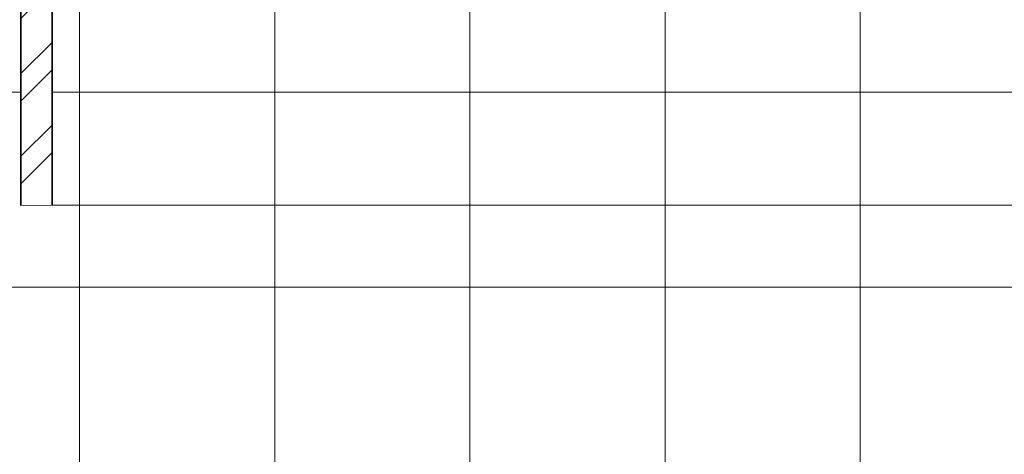
# Model space of a CAD drawing. Units: inches. Extents: x 351 to 1738, y -265 to 286.
# Tile 32 of 38: x 1380 to 1506, y -35 to 20. Entities that reach past the tile are written whole.
import ezdxf

# ---------------------------------------------------------------- set-up
doc = ezdxf.new("R2010")
doc.units = ezdxf.units.IN
doc.header["$MEASUREMENT"] = 0
for name, color, linetype, lineweight in [('A-ANNO-DIMS', 2, 'Continuous', 18), ('A-DOOR', 3, 'Continuous', 18), ('A-FLOR-PATT', 9, 'Continuous', 9), ('A-WALL', 7, 'Continuous', 35), ('A-WALL-PATT', 152, 'Continuous', 13)]:
    doc.layers.add(name, color=color, linetype=linetype, lineweight=lineweight)
doc.styles.get("Standard").update_dxf_attribs({"font": 'arial.ttf'})
doc.dimstyles.get("Standard").update_dxf_attribs({"dimtxt": 8, "dimasz": 5, "dimexe": 0.18, "dimexo": 0.0625, "dimgap": 0.09, "dimtad": 1, "dimtoh": 1, "dimzin": 0, "dimdsep": 46, "dimlunit": 4, "dimtxsty": 'Standard', "dimcen": 0, "dimclre": 256, "dimadec": 0, "dimazin": 0, "dimtfac": 1, "dimtofl": 0, "dimtmove": 0, "dimatfit": 3, "dimfxl": 1, "dimtolj": 1, "dimtzin": 0, "dimlwe": -1, "dimarcsym": 0})

# ---------------------------------------------------------------- blocks, each defined once
blk = doc.blocks.new('*D66')
at = {"layer": 'A-ANNO-DIMS', "transparency": 16777216}
for p, q in [((1384.27, -3.5), (1596.33, -3.5)), ((1384.27, -45), (1596.33, -45))]:
    blk.add_line(p, q, dxfattribs=at)
at = {"layer": 'A-ANNO-DIMS', "color": 0, "lineweight": -2, "transparency": 16777216}
blk.add_line((1596.15, -40), (1596.15, -8.5), dxfattribs=at)
at = {"layer": 'A-ANNO-DIMS', "color": 0, "transparency": 16777216}
for points in [[(1595.32, -8.5), (1596.99, -8.5), (1596.15, -3.5)], [(1595.32, -40), (1596.99, -40), (1596.15, -45)]]:
    blk.add_solid(points, dxfattribs=at)
at = {"layer": 'Defpoints', "color": 0, "transparency": 16777216}
for p in [(1384.2, -3.5), (1596.15, -3.5), (1384.2, -45)]:
    blk.add_point(p, dxfattribs=at)
at = {"layer": 'A-ANNO-DIMS', "color": 0, "transparency": 16777216, "insert": (1591.92, -24.25), "char_height": 8, "attachment_point": 5, "rotation": 90}
blk.add_mtext('\\A1;3\'-5 1/2"', dxfattribs=at)

msp = doc.modelspace()

# ---------------------------------------------------------------- hatches: boundary and pattern name
at = {"layer": 'A-FLOR-PATT', "transparency": 33554559}
h = msp.add_hatch(dxfattribs=at)
h.set_pattern_fill('ANSI37', color=256, scale=200, angle=135)
h.set_pattern_definition([(180, (1112.704, -164.037), (-2e-15, -25), []), (270, (1112.704, -164.037), (25, -5e-15), [])])
h.paths.add_polyline_path([(1380.064, 73.463), (1380.132, 148.463), (1338.064, 148.463), (1290.704, 148.463), (1290.704, 88.463), (1248.704, 88.463), (1248.704, -2.009), (1244.704, -2.009), (1244.704, 142.457), (1160.704, 142.457), (1160.704, 158.963), (1160.704, 170.137), (1160.704, 206.137), (1160.704, 228.963), (1112.704, 228.963), (1112.704, 209.963), (1112.704, 168.963), (1124.704, 168.963), (1124.704, 162.963), (1112.704, 162.963), (1112.704, 64.463), (1112.704, 60.463), (1112.704, 0.463), (1112.704, -48.026), (1146.804, -47.981), (1146.804, -35.691), (1207.804, -35.691), (1207.804, -47.902), (1236.542, -47.864), (1236.544, -50.009), (1248.5, -50.009), (1248.506, -102.915), (1248.512, -150.915), (1248.514, -164.037), (1248.549, -164.037), (1273.017, -164.037), (1273.017, -128.799), (1355.24, -128.799), (1355.24, -164.037), (1384.204, -164.037), (1384.204, -57.037), (1380.064, -57.037), (1380.064, -48.037), (1392.064, -48.037), (1392.064, -53.037), (1406.549, -53.037), (1406.549, -57.037), (1401.204, -57.037), (1401.204, -147.037), (1468.204, -147.037), (1468.204, -138.5), (1472.204, -138.5), (1472.204, -102.5), (1468.204, -102.5), (1468.204, -57.037), (1442.549, -57.037), (1442.549, -53.037), (1463.049, -53.037), (1463.049, -40.747), (1524.049, -40.747), (1524.049, -48.037), (1536.064, -48.037), (1536.064, -53.037), (1557.704, -53.037), (1557.704, 204.963), (1384.204, 204.963), (1384.204, 73.463), (1392.064, 73.463), (1392.064, 64.463), (1384.204, 64.463), (1384.204, -3.5), (1380.204, -3.537), (1380.204, 64.463), (1380.064, 64.463)])
h.paths.add_polyline_path([(1510.714, 86.458, -0.1039845), (1511.661, 85.595, 0.4704384), (1510.158, 87.614, 0.0961001)], flags=16)
h.paths.add_polyline_path([(1510.443, 100.266, 0.009798), (1504.693, 100.48, 0.0287898), (1504.6, 99.767, -0.1653311), (1505.519, 96.135, -0.1436014)], flags=16)
h.paths.add_polyline_path([(1487.201, 85.595, -0.1039845), (1488.148, 86.458, 0.0961001), (1488.704, 87.614, 0.4704384)], flags=0)
h.paths.add_polyline_path([(1495.052, 100.43), (1494.178, 100.43, -0.0264629), (1494.262, 99.774, -0.1442193)], flags=16)
h.paths.add_polyline_path([(1444.485, 86.458, -0.1039845), (1445.433, 85.595, 0.4704384), (1443.93, 87.614, 0.0961001)], flags=16)
h.paths.add_polyline_path([(1420.972, 85.595, -0.1039845), (1421.92, 86.458, 0.0961001), (1422.475, 87.614, 0.4704384)], flags=16)
h.paths.add_polyline_path([(1428.632, 100.335, 0.0010541), (1427.971, 100.309, -0.0215241), (1428.033, 99.774, -0.1143008)], flags=16)
h.paths.add_polyline_path([(1419.906, 143.708, 0.0249793), (1420.222, 157.526), (1421.573, 159.101), (1421.573, 175.369), (1391.393, 175.369), (1391.393, 200.519), (1542.294, 200.519), (1542.294, 175.369), (1512.028, 175.369, 0.0198653), (1511.521, 153.838, 0.0251335), (1512.758, 118.323, 0.0205529), (1512.942, 115.253), (1419.834, 115.253, -0.0004142), (1419.843, 124.798), (1413.059, 124.798), (1413.059, 84.437, -0.0618528), (1415.831, 80.45, -0.0930773), (1420.972, 85.595, -0.2675367), (1422.371, 84.732, 0.0851103), (1424.052, 84.616, -0.8853927), (1424.033, 84.851, -1.1258145), (1424.073, 84.366, -0.0879871), (1422.371, 84.732, -0.2675367), (1422.326, 83.089, -0.3705421), (1420.972, 85.595, 0.0930773), (1415.831, 80.45, -0.0874142), (1417.914, 73.937), (1418.941, 73.937, 0.0272504), (1418.913, 76.906, -0.1157032), (1421.051, 73.937), (1445.354, 73.937, -0.1157032), (1447.492, 76.906, 0.0272504), (1447.464, 73.937), (1448.491, 73.937, -0.0874142), (1450.574, 80.45, 0.0930773), (1445.433, 85.595, -0.3705421), (1444.079, 83.089, -0.2675367), (1444.034, 84.732, -0.0879871), (1442.332, 84.366, -1.1258145), (1442.372, 84.851, -2.0327363), (1442.364, 84.368, 0.0863779), (1444.034, 84.732, -0.2675367), (1445.433, 85.595, -0.0930773), (1450.574, 80.45, -0.2577317), (1466.483, 90.927, -0.4786702), (1468.832, 91.907, -0.4786702), (1471.18, 90.927, -0.26264), (1483.053, 81.78, -0.0718662), (1487.201, 85.595, -0.2675367), (1488.6, 84.732, 0.0851103), (1490.28, 84.616, -0.8853927), (1490.262, 84.851, -1.1258145), (1490.301, 84.366, -0.0879871), (1488.6, 84.732, -0.2675367), (1488.554, 83.089, -0.3705421), (1487.201, 85.595, 0.0718662), (1483.053, 81.78, -0.1320648), (1484.143, 73.937), (1485.169, 73.937, 0.0272504), (1485.142, 76.906, -0.1157032), (1487.28, 73.937), (1511.582, 73.937, -0.1157032), (1513.72, 76.906, 0.0272504), (1513.693, 73.937), (1514.719, 73.937, -0.0874142), (1516.802, 80.45, 0.0930773), (1511.661, 85.595, -0.3705421), (1510.308, 83.089, -0.2675367), (1510.262, 84.732, -0.0879871), (1508.561, 84.366, -1.1258145), (1508.601, 84.851, -2.0327363), (1508.592, 84.368, 0.0863779), (1510.262, 84.732, -0.2675367), (1511.661, 85.595, -0.0930773), (1516.802, 80.45, -0.0618528), (1519.575, 84.437), (1519.575, 73.937), (1413.059, 73.937), (1413.059, 124.798), (1419.843, 124.798, -0.0008205)], flags=16)
h.paths.add_polyline_path([(1220.149, 54.133, -0.1039845), (1220.869, 53.476, 0.4704384), (1219.727, 55.011, 0.0961001)], flags=16)
h.paths.add_polyline_path([(1219.944, 64.626, 0.009798), (1215.574, 64.789, 0.0287898), (1215.503, 64.247, -0.1653311), (1216.201, 61.487, -0.1436014)], flags=16)
h.paths.add_polyline_path([(1209.779, 64.449, 0.0974459), (1209.339, 64.751), (1208.247, 64.751, 0.1273905), (1207.7, 64.326, 0.1715858), (1206.95, 61.475, -0.1588542), (1207.636, 59.45, 0.0158984), (1207.795, 59.218, 0.0615457), (1208.598, 59.616, 0.1754158), (1208.638, 60.099, -0.2847793), (1209.348, 62.472, 0.3262165)], flags=16)
h.paths.add_polyline_path([(1169.818, 54.133, -0.1039845), (1170.538, 53.476, 0.4704384), (1169.396, 55.011, 0.0961001)], flags=16)
h.paths.add_polyline_path([(1159.017, 62.472, 0.2847642), (1158.307, 60.099, -0.1754332), (1158.267, 59.616, 0.3929302), (1159.448, 64.449, -0.3262298)], flags=16)
h.paths.add_polyline_path([(1156.342, 58.239, -0.1783213), (1154.011, 55.31, -0.1747359), (1154.722, 55.233, -0.2008015), (1156.27, 56.086, 0.1269899), (1157.283, 58.991, -0.0912053)], flags=16)
h.paths.add_polyline_path([(1156.624, 61.413, 0.1572752), (1157.316, 64.247, 0.1696217)], flags=16)
h.paths.add_polyline_path([(1152.67, 54.133, -0.0961001), (1151.95, 53.476, 0.0640762), (1154.465, 54.384, 0.1990158)], flags=16)
h.paths.add_polyline_path([(1202.281, 53.476, -0.1039845), (1203, 54.133, 0.0961001), (1203.423, 55.011, 0.4704384)], flags=0)
h.paths.add_polyline_path([(1151.139, 97.64, 0.0249793), (1151.379, 108.141), (1152.406, 109.338), (1152.406, 121.701), (1129.47, 121.701), (1129.47, 140.814), (1244.149, 140.814), (1244.149, 121.701), (1221.148, 121.701, 0.0198653), (1220.763, 105.338, 0.0251335), (1221.703, 78.349, 0.0205529), (1221.843, 76.016), (1151.078, 76.016, -0.1287433), (1148.786, 65.037, 0.5393525), (1150.327, 64.171, -0.027594), (1163.481, 64.751, 0.0976954), (1163.04, 64.449, 0.3262165), (1163.471, 62.472, -0.2847765), (1164.181, 60.099, -0.1947567), (1165.846, 61.443, -0.1554021), (1165.172, 64.247, -0.1660224), (1165.869, 61.475, -0.1770142), (1167.852, 62.77, -0.4482027), (1169.974, 60.807, -0.3934987), (1167.679, 57.86, -0.8955483), (1168.438, 54.524, -0.3557668), (1166.218, 56.086, -0.066024), (1165.505, 57.539), (1165.251, 56.243, -0.3717324), (1164.02, 59.758, -0.3736141), (1163.04, 64.449, -0.0976954), (1163.481, 64.751, 0.0213538), (1153.294, 64.429, -0.1341826), (1156.695, 61.368, 0.1868727), (1154.636, 62.77, 0.4482027), (1152.514, 60.807, 0.4037263), (1154.905, 57.846, 0.7112192), (1153.334, 55, 0.5315397), (1151.95, 53.476, -0.2675367), (1153.013, 52.821, 0.0851103), (1154.29, 52.732, -0.8853927), (1154.276, 52.911, -1.1258145), (1154.306, 52.543, -0.0879871), (1153.013, 52.821, -0.2675367), (1152.978, 51.572, -0.3705421), (1151.95, 53.476, 0.0930773), (1148.043, 49.566, -0.0874142), (1149.626, 44.617), (1150.406, 44.617, 0.0272504), (1150.385, 46.873, -0.1157032), (1152.01, 44.617), (1170.478, 44.617, -0.1157032), (1172.103, 46.873, 0.0272504), (1172.082, 44.617), (1172.862, 44.617, -0.0874142), (1174.445, 49.566, 0.0930773), (1170.538, 53.476, -0.3705421), (1169.51, 51.572, -0.2675367), (1169.475, 52.821, -0.0879871), (1168.182, 52.543, -1.1258145), (1168.212, 52.911, -2.0327363), (1168.206, 52.544, 0.0863779), (1169.475, 52.821, -0.2675367), (1170.538, 53.476, -0.0930773), (1174.445, 49.566, -0.2577317), (1186.536, 57.528, -0.4786702), (1188.321, 58.273, -0.4786702), (1190.106, 57.528, -0.26264), (1199.128, 50.577, -0.0718662), (1202.281, 53.476, -0.2675367), (1203.344, 52.821, 0.0851103), (1204.621, 52.732, -0.8853927), (1204.607, 52.911, -1.1258145), (1204.637, 52.543, -0.0879871), (1203.344, 52.821, -0.2675367), (1203.309, 51.572, -0.3705421), (1202.281, 53.476, 0.0718662), (1199.128, 50.577, -0.1320648), (1199.957, 44.617), (1200.737, 44.617, 0.0272504), (1200.716, 46.873, -0.1157032), (1202.341, 44.617), (1220.809, 44.617, -0.1157032), (1222.434, 46.873, 0.0272504), (1222.413, 44.617), (1223.193, 44.617, -0.0874142), (1224.776, 49.566, 0.0930773), (1220.869, 53.476, -0.3705421), (1219.841, 51.572, -0.2675367), (1219.806, 52.821, -0.0879871), (1218.513, 52.543, -1.1258145), (1218.543, 52.911, -2.0327363), (1218.537, 52.544, 0.0863779), (1219.806, 52.821, -0.2675367), (1220.869, 53.476, -0.0930773), (1224.776, 49.566, -0.0618528), (1226.883, 52.597), (1226.883, 44.617), (1145.936, 44.617), (1145.936, 83.269), (1151.091, 83.269, -0.0008205)], flags=16)
h.paths.add_polyline_path([(1218.01, 57.86, -0.8955483), (1218.769, 54.524, -0.3557668), (1216.549, 56.086, -0.066024), (1215.836, 57.539), (1215.582, 56.243, -0.3717324), (1214.351, 59.758, -0.3736141), (1213.371, 64.449, 0.3262165), (1213.802, 62.472, -0.2847765), (1214.512, 60.099, -0.1947567), (1216.177, 61.443, -0.1799907), (1218.183, 62.77, -0.4482027), (1220.305, 60.807, -0.3934987)], flags=16)
h.paths.add_polyline_path([(1424.735, 91.363, -0.3934987), (1421.715, 95.241, -0.4482027), (1424.507, 97.824, -0.1799907), (1427.147, 96.077, -0.1947567), (1429.338, 94.309, -0.2847765), (1430.272, 97.432, 0.3262165), (1430.839, 100.034, -0.3736141), (1429.55, 93.861, -0.3717324), (1427.929, 89.235), (1427.596, 90.941, -0.066024), (1426.657, 89.029, -0.3557668), (1423.736, 86.973, -0.8955483)], flags=16)
h.paths.add_polyline_path([(1238.033, 131.257, -1), (1227.329, 131.257, -1)], flags=0)
h.paths.add_polyline_path([(1235.357, 131.257, -1), (1230.005, 131.257, -1)], flags=0)
h.paths.add_polyline_path([(1214.039, 54.243, 0.1543819), (1214.38, 53.992, 0.3589549), (1213.613, 54.016, 0.6039484), (1214.379, 53.657, 0.3713191), (1213.968, 52.872, 0.1879935), (1214.312, 52.809, -0.592455), (1213.953, 52.967, -0.2942791), (1214.083, 53.691, -1.3001871), (1213.881, 54.134, -0.2837621), (1214.469, 53.896, 1.1509396)], flags=16)
h.paths.add_polyline_path([(1212.091, 56.286, -0.4084338), (1211.337, 56.445, -0.0362594), (1211.098, 56.848, -0.2360976), (1211.59, 56.63, 0.0353445), (1211.835, 56.543, -0.4752408), (1212.091, 56.286, -0.4752408), (1212.438, 56.182, 0.0353445), (1212.631, 56.007, -0.2360976), (1213.056, 55.676, -0.0362594), (1212.588, 55.697, -0.4084338)], flags=16)
h.paths.add_polyline_path([(1211.469, 50.297, 0.296043), (1210.47, 50.527, 0.310883), (1211.931, 50.148, 0.0212546)], flags=16)
h.paths.add_polyline_path([(1213.739, 51.818, -0.0362594), (1213.271, 51.838, -0.4084337), (1212.774, 52.427, -0.0947856), (1212.293, 50.703, 1.1504738), (1212.911, 50.232, 0.1662877), (1213.265, 50.68, -0.0252543), (1212.603, 50.13, 1.0879317), (1212.471, 49.407, 0.1662877), (1213.02, 49.251, -0.016128), (1212.567, 49.563, -0.286859), (1212.217, 49.638, 0.0221563), (1212.046, 50.055, -0.6461302), (1212.185, 50.498, 0.0884116), (1212.732, 52.077, -1.1860374), (1213.121, 52.323, 0.0353445), (1213.314, 52.148, -0.2360976)], flags=16)
h.paths.add_polyline_path([(1212.094, 50.342, -0.0485241), (1211.54, 49.605, -1.1038339), (1211.397, 48.738, -0.7855147), (1211.683, 48.254, -0.3920429), (1210.948, 48.525, -0.3928194), (1210.561, 47.995, -0.592455), (1210.201, 48.153, -0.2942791), (1210.331, 48.877, -0.7041716), (1210.316, 49.592, -0.6793441), (1210.729, 50.112, 0.5636764)], flags=16)
h.paths.add_polyline_path([(1211.274, 49.829, -0.1398258), (1210.745, 49.859, -0.2178785), (1210.948, 49.509, -0.4985724)], flags=0)
h.paths.add_polyline_path([(1433.426, 81.49, -0.181571), (1434.245, 81.788, -0.0080665), (1433.726, 82.205, 0.0455784), (1432.755, 81.242, 0.1790113)], flags=16)
h.paths.add_polyline_path([(1434.146, 81.009, -0.1324418), (1433.645, 80.771, 0.2590893), (1433.234, 80.471, -0.1802109), (1433.392, 80.805, -0.1699398), (1432.758, 81.109, 0.0326525), (1433.273, 80.474, -0.4933627), (1434.046, 80.146, -0.3904966)], flags=16)
h.paths.add_polyline_path([(1434.83, 80.047, -0.9475376), (1435.294, 79.576, -0.2991282), (1434.625, 79.404, -0.2704392), (1435.01, 78.591, -0.592455), (1434.537, 78.382, -0.3928194), (1434.027, 79.08, -0.3920429), (1433.06, 78.723, -0.3520423), (1433.003, 79.197, -0.1972159), (1433.75, 79.734, -0.7136405), (1434.447, 79.939, -0.2147903), (1434.819, 80.475, 0.4088333), (1435.075, 80.803, -0.2261519)], flags=16)
h.paths.add_polyline_path([(1432.67, 81.217, -0.4542182), (1431.897, 79.923, -0.4144105), (1431.301, 80.035, 0.0161291), (1431.897, 80.445, 0.2795702), (1432.073, 80.871, -0.2895037), (1431.103, 81.321, -0.4144105), (1430.978, 81.915, 0.0161296), (1431.586, 81.521, 0.341293), (1432.125, 81.583, -0.8131856)], flags=16)
h.paths.add_polyline_path([(1429.893, 86.381, -0.9475376), (1430.358, 85.91, -0.1731062), (1429.984, 85.712, -0.0388172), (1431.625, 84.214, -0.0879005), (1432.097, 88.549, -0.0497684), (1431.254, 88.49, -0.2360976), (1431.814, 88.925, 0.0353445), (1432.067, 89.155, -0.4752408), (1432.524, 89.291, -0.4752408), (1432.86, 89.63, 0.0353445), (1433.182, 89.744, -0.2360976), (1433.83, 90.032, -0.0362594), (1433.516, 89.502, -0.4084338), (1432.524, 89.291, -0.3124239), (1432.106, 88.58, 0.0885594), (1431.625, 84.214, -0.4084337), (1430.971, 83.439, -0.0362594), (1430.355, 83.412, -0.2360976), (1430.914, 83.847, 0.0353445), (1431.168, 84.078, -0.4752408), (1431.625, 84.214, 0.0388172), (1429.984, 85.712, -0.3217316), (1429.333, 86.048, -0.32743), (1429.883, 86.809, 0.4088333), (1430.138, 87.138, -0.2261519)], flags=16)
h.paths.add_polyline_path([(1211.206, 58.616, -0.9997836), (1211.336, 59.323, -0.6149935)], flags=16)
h.paths.add_polyline_path([(1210.288, 49.429, 0.1543819), (1210.629, 49.178, 0.3589549), (1209.861, 49.202, 0.6039484), (1210.627, 48.843, -0.5348247), (1210.806, 49.295, 0.7483464)], flags=16)
h.paths.add_polyline_path([(1209.589, 51.828, -0.0087906), (1209.775, 51.753, 0.1122315), (1209.466, 52.019, 1.4188509), (1209.014, 51.708, -0.4587257), (1208.651, 51.073, -0.592455), (1208.291, 51.232, -0.2942791), (1208.421, 51.955, -1.3001871), (1208.219, 52.398, -0.2260052), (1208.719, 52.257, -0.4755189), (1209.158, 52.369, -1.4554994), (1209.603, 52.664, 0.4213049), (1209.191, 52.262, -0.5912116), (1208.979, 51.796, 0.4973986), (1209.773, 51.333, 0.6493116)], flags=16)
h.paths.add_polyline_path([(1208.029, 52.041, 0.5446671), (1208.832, 52.045, 0.220132)], flags=0)
h.paths.add_polyline_path([(1210.438, 51.425, -0.2041997), (1210.277, 52.018, 0.2708262), (1209.915, 52.897, 0.3241145)], flags=0)
h.paths.add_polyline_path([(1209.668, 52.407, -0.60139), (1208.99, 52.221, -0.3949159), (1208.248, 52.83, -0.8367916), (1208.651, 53.017, -0.3384876), (1209.039, 52.571, 0.1941379), (1209.191, 52.262, 0.4139945), (1209.712, 52.475, 0.5177103), (1210.503, 51.416, 0.401922), (1209.493, 50.93, 0.2063956), (1209.516, 50.165, -0.3194629), (1210.417, 51.418, -0.466635)], flags=16)
h.paths.add_polyline_path([(1206.601, 56.086, -0.3557668), (1204.381, 54.524, -0.9211983), (1205.236, 57.846, 0.2065693), (1207.614, 58.991, -0.1269899)], flags=16)
h.paths.add_polyline_path([(1435.487, 82.816, 0.5277653), (1436.615, 83.361, 0.5085402), (1437.05, 82.433, 0.592455), (1437.524, 82.641, 0.3312448), (1436.963, 83.548, 0.3878632), (1437.808, 83.626, 0.5929544), (1437.618, 84.176, 0.2260158), (1436.961, 83.99, 0.3182053), (1437.588, 84.854, 0.6893744), (1437.05, 84.991, 0.3357648), (1436.539, 84.41, -0.1569934), (1436.404, 84.065, -0.4346112), (1436.961, 83.99, -0.2147903), (1437.333, 84.526, 0.4088333), (1437.588, 84.854, -0.2261519), (1437.343, 84.097, -0.9475376), (1437.808, 83.626, -0.2991282), (1437.139, 83.455, -0.2704392), (1437.524, 82.641, -0.592455), (1437.05, 82.433, -0.3928194), (1436.541, 83.13, -0.4396601), (1435.475, 82.794, -0.174614), (1435.942, 82.244, -0.2063956), (1435.912, 81.237, -0.2708262), (1435.125, 82.208, 0.2079765), (1434.686, 82.904, -0.1964955)], flags=16)
h.paths.add_polyline_path([(1435.386, 84.832, 0.270811), (1434.91, 83.676, -0.2042174), (1434.699, 82.895, 0.3241145)], flags=0)
h.paths.add_polyline_path([(1435.68, 84.18, -0.2176564), (1435.554, 83.304, -0.1767045), (1436.236, 83.778, -0.3730364)], flags=0)
h.paths.add_polyline_path([(1435.566, 100.034, 0.3262165), (1436.133, 97.432, -0.2847765), (1437.067, 94.309, -0.1947567), (1439.258, 96.077, -0.1554021), (1438.371, 99.767, -0.1660224), (1439.289, 96.12, -0.1770142), (1441.897, 97.824, -0.4482027), (1444.69, 95.241, -0.3934987), (1441.67, 91.363, -0.8955483), (1442.669, 86.973, -0.3557668), (1439.748, 89.029, -0.066024), (1438.809, 90.941), (1438.476, 89.235, -0.3717324), (1436.855, 93.861, -0.3736141)], flags=16)
h.paths.add_polyline_path([(1191.252, 49.507, -0.2740221), (1190.658, 48.409, 0.2675367), (1191.311, 47.344, 0.3705421)], flags=0)
h.paths.add_polyline_path([(1190.301, 49.717, 0.1990158), (1188.619, 49.04, 0.0640762), (1191.252, 49.507, -0.0961001)], flags=0)
h.paths.add_polyline_path([(1189.518, 47.857, 1.1258145), (1189.676, 47.523, 2.0446052)], flags=0)
h.paths.add_polyline_path([(1464.974, 80.372, 0.2740221), (1465.756, 78.927, -0.0830131)], flags=0)
h.paths.add_polyline_path([(1464.974, 80.372, 0.3705421), (1464.897, 77.525, 0.5763244)], flags=0)
h.paths.add_polyline_path([(1464.974, 80.372, -0.4704384), (1467.284, 81.372, -0.0961001), (1466.226, 80.648, -0.1990158), (1468.439, 79.757, -0.0640762)], flags=0)
h.paths.add_polyline_path([(1189.511, 56.43, -0.2594668), (1188.321, 56.391, -0.2594668), (1187.13, 56.43, 0.0851103), (1188.193, 55.716, -0.8853927), (1188.27, 55.878, -1.1960133), (1188.355, 55.442, 0.1014587)], flags=0)
h.paths.add_polyline_path([(1188.321, 57.596, 0.0780722), (1187.678, 57.24, 0.0155503), (1188.321, 57.136, 0.0155503), (1188.964, 57.24, 0.0780722)], flags=0)
h.paths.add_polyline_path([(1190.164, 55.365, -0.5763244), (1190.106, 57.528, -0.1982945), (1188.321, 58.319, -0.1982945), (1186.536, 57.528, -0.5763244), (1186.477, 55.365, -0.3705421), (1186.536, 57.528, 0.1982945), (1188.321, 58.319, 0.1982945), (1190.106, 57.528, -0.3705421)], flags=0)
h.paths.add_polyline_path([(1188.372, 55.878, 1.1258145), (1188.529, 55.544, 2.0446052)], flags=0)
h.paths.add_polyline_path([(1186.341, 49.717, -0.0961001), (1185.389, 49.507, 0.0640762), (1188.022, 49.04, 0.1990158)], flags=0)
h.paths.add_polyline_path([(1185.389, 49.507, -0.2675367), (1185.984, 48.409, 0.0851103), (1187.046, 47.695, -0.8853927), (1187.123, 47.857, -1.1258145), (1186.966, 47.523, -0.0879871), (1185.984, 48.409, -0.2675367), (1185.331, 47.344, -0.3705421)], flags=0)
h.paths.add_polyline_path([(1399.441, 187.944, -1), (1413.525, 187.944, -1)], flags=0)
h.paths.add_polyline_path([(1402.962, 187.944, -1), (1410.004, 187.944, -1)], flags=0)
h.paths.add_polyline_path([(1357.663, -72.245), (1377.272, -72.245), (1377.272, -91.854), (1357.663, -91.854)], flags=16)
h.paths.add_polyline_path([(1467.256, 78.201, -1.1258145), (1467.049, 77.761, -2.0446052)], flags=0)
h.paths.add_polyline_path([(1468.822, 88.714, 0.9411249), (1469.106, 88.316, 1.1371523), (1468.765, 88.755, 0.890986), (1468.99, 88.245, 0.0948283), (1470.398, 89.481, -0.2675367), (1471.18, 90.927, -0.0281232), (1469.678, 90.547, -0.0287737), (1469.948, 90.311, -0.0203267), (1468.832, 90.41, -0.0203267), (1467.716, 90.311, -0.0287737), (1467.986, 90.547, -0.0281232), (1466.483, 90.927, -0.2675367), (1467.265, 89.481, 0.0851103), (1468.663, 88.542, -1.2023159)], flags=0)
h.paths.add_polyline_path([(1178.25, 124.523, -0.1199286), (1165.65, 124.145, -0.1073492), (1159.133, 124.446, -0.1028906), (1159.132, 130.465, -0.0748968), (1158.993, 137.956, 0.002027), (1167.844, 137.479, -0.07553), (1180.337, 137.666, -0.0758613), (1186.502, 137.688, -0.1409896), (1186.272, 130.046, -0.0954805), (1186.729, 124.748, -0.10603)], flags=0)
h.paths.add_polyline_path([(1469.225, 79.757, -0.1990158), (1471.437, 80.648, -0.0961001), (1470.379, 81.372, -0.4704384), (1472.689, 80.372, -0.3705421), (1472.766, 77.525, -0.2675367), (1471.907, 78.927, -0.0879863), (1470.615, 77.761, -1.1258491), (1470.408, 78.201, -2.0327363), (1470.642, 77.778, 0.0863779), (1471.907, 78.927, -0.2675367), (1472.689, 80.372, -0.0640762)], flags=0)
h.paths.add_polyline_path([(1430.423, 186.902, -0.0748968), (1430.24, 196.758, 0.002027), (1441.887, 196.131, -0.07553), (1458.326, 196.377, -0.0758613), (1466.438, 196.406, -0.1409896), (1466.136, 186.35, -0.0954805), (1466.737, 179.378, -0.10603), (1455.58, 179.082, -0.1199286), (1439, 178.585, -0.1073492), (1430.425, 178.981, -0.1028906)], flags=0)
h.paths.add_polyline_path([(1162.258, 49.939, 0.3357645), (1161.87, 49.497, -0.1569936), (1161.767, 49.235, -0.4346112), (1162.19, 49.178, -0.2147903), (1162.473, 49.585, 1.5291948)], flags=16)
h.paths.add_polyline_path([(1161.683, 49.021, 0.5815181), (1161.268, 49.583, 0.5927609)], flags=16)
h.paths.add_polyline_path([(1162.602, 48.058, 0.3713191), (1162.192, 48.843, 0.4345332), (1162.88, 48.962, 0.1850806), (1162.197, 48.926, 1.1218369)], flags=16)
h.paths.add_polyline_path([(1161.443, 48.941, -1.3071038), (1161.495, 48.571, -0.2177521), (1161.136, 48.254, 0.6973029), (1161.871, 49.048, 0.1215141)], flags=16)
h.paths.add_polyline_path([(1162.531, 49.429, -0.2070837), (1162.05, 49.146, -0.9920299)], flags=16)
h.paths.add_polyline_path([(1161.304, 49.578, -0.7196675), (1161.513, 50.079, -0.1304275), (1160.836, 50.168, 0.0395926)], flags=0)
h.paths.add_polyline_path([(1162.036, 50.584, -0.0080665), (1161.642, 50.9, 0.0293675), (1161.35, 50.297, -0.2057884)], flags=16)
h.paths.add_polyline_path([(1162.882, 51.392, -0.1247327), (1162.763, 51.828, -0.1011907), (1162.399, 51.438, -0.153425)], flags=0)
h.paths.add_polyline_path([(1164.235, 51.85, -0.3091075), (1164.513, 51.136, -0.6271245), (1163.781, 51.603, -0.6859091), (1162.777, 51.219, -0.2332851), (1163.303, 50.165, -0.2708262), (1162.705, 50.903, 0.2041997), (1162.381, 51.425, 0.204182), (1162.542, 52.018, -0.2708414), (1162.903, 52.897, -0.1272607), (1163.219, 52.529, -1.1686811), (1163.781, 52.587, -0.3291117), (1164.168, 53.017, -0.8367917), (1164.571, 52.83, -0.1933406), (1164.391, 52.338, -0.9475376), (1164.744, 51.981, -0.2991282)], flags=16)
h.paths.add_polyline_path([(1163.598, 51.937, -1.2629561), (1163.236, 51.831, 0.0125754), (1162.971, 51.721, 0.2306566), (1163.151, 52.407, -0.1648982), (1163.178, 52.661, -0.4493201), (1163.628, 52.262, -0.721477), (1164.154, 52.088, -0.8499982)], flags=0)
h.paths.add_polyline_path([(1161.613, 58.616, -0.9804131), (1161.525, 59.049, -2.9089348)], flags=16)
h.paths.add_polyline_path([(1160.252, 49.166, -0.4144105), (1159.799, 49.251, 0.0161291), (1160.252, 49.563, 0.2795702), (1160.386, 49.887, -0.2895037), (1159.649, 50.229, -0.4144105), (1159.554, 50.68, 0.0161296), (1160.015, 50.381, 0.6178854), (1160.526, 50.703, -0.0947856), (1160.045, 52.427, -0.1404436), (1159.682, 52.042, -0.0578559), (1159.3, 51.872, 0.5448433), (1160.046, 52.419, -0.0881216), (1160.404, 55.721, -0.0497684), (1159.763, 55.676, -0.2360976), (1160.188, 56.007, 0.0353445), (1160.381, 56.182, -0.4752408), (1160.728, 56.286, -0.4752408), (1160.984, 56.543, 0.0353445), (1161.229, 56.63, -0.2360976), (1161.721, 56.848, -0.0362594), (1161.482, 56.445, -0.4084338), (1160.728, 56.286, -0.3124239), (1160.411, 55.745, 0.0885594), (1160.045, 52.427, 0.1070813), (1160.634, 50.498, -0.4947977), (1160.839, 50.149, -0.4542182)], flags=16)
h.paths.add_polyline_path([(1160.666, 49.808, -2.0765276), (1160.828, 50.172, 0.0195861)], flags=0)
h.paths.add_polyline_path([(1158.439, 53.992, 0.1543819), (1158.78, 54.243, 0.7483463), (1158.262, 54.109, -0.3382251), (1158.492, 53.839, -0.1708158), (1159.124, 53.779, 0.4957286), (1158.938, 54.134, 0.2260157)], flags=16)
h.paths.add_polyline_path([(1160.045, 52.427, 0.0388172), (1158.798, 53.565, -0.1198178), (1158.574, 53.586, -0.3091075), (1158.851, 52.872, -0.1879935), (1158.506, 52.809, 0.592455), (1158.866, 52.967, 0.3312448), (1158.44, 53.657, 0.2012451), (1158.798, 53.565, -0.034023), (1159.901, 52.578, -0.0442527), (1159.698, 52.323, -0.4752408)], flags=16)
h.paths.add_polyline_path([(1336.926, -95.392), (1336.926, -117.945), (1291.82, -117.945), (1291.82, -95.392)], flags=16)
h.paths.add_polyline_path([(1357.535, -97.244), (1357.726, -96.697, 0.0348443)], flags=16)
h.paths.add_polyline_path([(1376.693, -96.478), (1377.301, -96.5, 0.0314968), (1375.907, -96.424), (1357.726, -96.424)], flags=16)
h.paths.add_polyline_path([(1379.403, -119.667, 0.0267056), (1380.043, -119.439, -0.0152991)], flags=16)
h.paths.add_polyline_path([(1357.726, -120.202), (1357.821, -120.202), (1357.821, -120.201)], flags=16)
h.paths.add_polyline_path([(1354.171, -104.592), (1354.469, -98.672, 0.0111377)], flags=16)
h.paths.add_polyline_path([(1355.058, -119.136), (1354.578, -118.539, 0.1431635)], flags=16)
h.paths.add_polyline_path([(1378.851, -96.821), (1378.85, -96.82), (1378.85, -96.82, -0.0496798), (1380.055, -97.191), (1378.85, -96.82, 0.1500541), (1375.135, -97.188), (1375.136, -119.44, -0.0099698), (1374.747, -116.649), (1357.726, -116.649, 0.1693849), (1357.535, -119.382), (1357.535, -119.382), (1357.535, -119.382, 0.0348176), (1357.726, -119.928), (1357.726, -119.928), (1357.726, -119.929, -0.0348772), (1357.535, -119.382), (1355.507, -119.382), (1355.317, -119.278), (1357.535, -119.382, -0.1693939), (1357.726, -116.649, -0.0391513), (1374.686, -116.113, -0.0020149), (1374.625, -115.546, 0.1153223), (1369.915, -115.474, 0.0609215), (1369.922, -101.154, 0.1151459), (1374.625, -101.079, -0.0020164), (1374.686, -100.513, -0.0391511), (1357.726, -99.977), (1374.747, -99.977, -0.0099633), (1375.135, -97.188), (1375.135, -97.188, -0.1501081)], flags=16)
h.paths.add_polyline_path([(1490.963, 91.363, -0.3934987), (1487.944, 95.241, -0.4482027), (1490.736, 97.824, -0.1799907), (1493.376, 96.077, -0.1947567), (1495.567, 94.309, -0.2847765), (1496.501, 97.432, 0.3262165), (1497.068, 100.034, -0.3736141), (1495.778, 93.861, -0.3717324), (1494.158, 89.235), (1493.824, 90.941, -0.066024), (1492.886, 89.029, -0.3557668), (1489.964, 86.973, -0.8955483)], flags=16)
h.paths.add_polyline_path([(1354.86, -97.658), (1355.316, -97.348, 0.1019112)], flags=16)
h.paths.add_polyline_path([(1497.063, 83.327, 0.1767244), (1496.37, 83.785, -0.4051388), (1496.016, 83.384, 0.4973986), (1497.06, 82.774, 0.6493116), (1496.818, 83.426, -0.0087906)], flags=16)
h.paths.add_polyline_path([(1496.339, 83.783, 0.5927609), (1496.886, 84.522, 0.5815181)], flags=16)
h.paths.add_polyline_path([(1495.11, 82.641, 0.592455), (1495.583, 82.433, 0.6769152), (1495.805, 83.59, 0.3756693)], flags=16)
h.paths.add_polyline_path([(1495.015, 84.176, -0.145057), (1495.301, 84.526, -0.4088333), (1495.045, 84.854, 0.2206292), (1495.381, 84.152, -0.199594), (1495.851, 83.764, -0.5240172), (1494.826, 83.626, -0.5929976)], flags=16)
h.paths.add_polyline_path([(1501.655, 81.915, -0.0161291), (1501.048, 81.521, -0.3927187), (1500.462, 81.37, -0.2106699), (1500.607, 81.142, 0.3066994)], flags=16)
h.paths.add_polyline_path([(1500.11, 89.291, -0.4084338), (1499.118, 89.502, -0.0362594), (1498.803, 90.032, -0.2360976), (1499.451, 89.744, 0.0353445), (1499.774, 89.63, -0.4752408), (1500.11, 89.291, -0.4752408), (1500.567, 89.155, 0.0353445), (1500.82, 88.925, -0.2360976), (1501.379, 88.49, -0.0362594), (1500.763, 88.516, -0.4084338)], flags=16)
h.paths.add_polyline_path([(1498.908, 82.205, -0.0513217), (1500.013, 81.134, -0.5879306), (1500.234, 81.676, 0.1070813), (1501.009, 84.214, -0.03529)], flags=16)
h.paths.add_polyline_path([(1496.93, 83.875, -0.2063956), (1497.247, 84.832, -0.2708262), (1497.724, 83.676, 0.2079765), (1497.944, 82.884, -0.3814554)], flags=16)
h.paths.add_polyline_path([(1496.721, 81.237, 0.2708125), (1497.509, 82.208, -0.2042157), (1497.935, 82.895, 0.3241145)], flags=16)
h.paths.add_polyline_path([(1497.529, 80.125, -0.145057), (1497.814, 80.475, -0.703182), (1498.282, 81.178, -0.1229248), (1497.977, 81.714, -0.2708368), (1499.207, 81.49, 0.2079641), (1499.993, 81.248, -0.2651454), (1499.278, 80.472, 0.3819006), (1498.808, 79.947, -0.3059049), (1498.848, 79.519, 0.4994816), (1498.574, 79.217, -0.4587257), (1498.097, 78.382, -0.592455), (1497.624, 78.591, -0.2704392), (1498.009, 79.404, -0.299116), (1497.34, 79.576, -0.5930157)], flags=16)
h.paths.add_polyline_path([(1500.736, 79.923, 0.4144105), (1501.333, 80.035, -0.3216484), (1500.192, 80.765, 0.0198856), (1499.976, 81.251, 0.4653307)], flags=16)
h.paths.add_polyline_path([(1501.009, 84.214, -0.0388172), (1502.649, 85.712, -0.1730946), (1502.276, 85.91, -0.5930157), (1502.465, 86.46, -0.145057), (1502.751, 86.809, -0.4088333), (1502.495, 87.138, 0.2206292), (1502.831, 86.436, -0.199594), (1503.301, 86.048, -0.3217316), (1502.649, 85.712, 0.0388172), (1501.009, 84.214, 0.1224486), (1501.412, 83.755, 0.4754908), (1501.335, 84.226, 0.055822), (1501.719, 83.847, -0.2360976), (1502.278, 83.412, -0.0362594), (1501.663, 83.439, -0.4084338)], flags=16)
h.paths.add_polyline_path([(1501.794, 100.034, 0.3262165), (1502.362, 97.432, -0.2847765), (1503.295, 94.309, -0.1947567), (1505.486, 96.077, -0.1799907), (1508.126, 97.824, -0.4482027), (1510.918, 95.241, -0.3934987), (1507.899, 91.363, -0.8955483), (1508.898, 86.973, -0.3557668), (1505.976, 89.029, -0.066024), (1505.038, 90.941), (1504.704, 89.235, -0.3717324), (1503.084, 93.861, -0.3736141)], flags=16)
h.paths.add_polyline_path([(1146.29, 131.257, -1), (1135.587, 131.257, -1)], flags=0)
h.paths.add_polyline_path([(1143.614, 131.257, -1), (1138.262, 131.257, -1)], flags=0)
h.paths.add_polyline_path([(1524.064, 73.463), (1536.064, 73.463), (1536.064, 64.463), (1524.064, 64.463)], flags=16)
h.paths.add_polyline_path([(1520.162, 187.944, -1), (1534.246, 187.944, -1)], flags=0)
h.paths.add_polyline_path([(1530.725, 187.944), (1527.204, 187.944), (1527.204, 184.423, 0.4142136)], flags=0)
h.paths.add_polyline_path([(1278.415, -91.154), (1331.067, -91.154), (1331.067, -80.583), (1278.415, -80.583)], flags=24)
h.paths.add_polyline_path([(1266.655, -79.354), (1354.738, -79.354), (1354.738, -67.817), (1266.655, -67.817)], flags=24)
h.paths.add_polyline_path([(1115.482, 206.184), (1155.098, 206.184), (1155.098, 217.714), (1115.482, 217.714)], flags=24)
h.paths.add_polyline_path([(1161.771, 8.501), (1222.466, 8.501), (1222.466, 19.079), (1161.771, 19.079)], flags=24)
h.paths.add_polyline_path([(1164.656, 18.795), (1210.615, 18.795), (1210.615, 30.324), (1164.656, 30.324)], flags=24)
h.paths.add_polyline_path([(1368.147, -32.882), (1379.362, -32.882), (1379.362, -21.733), (1368.147, -21.733)], flags=24)
h.paths.add_polyline_path([(1244.842, -31.012), (1256.057, -31.012), (1256.057, -19.863), (1244.842, -19.863)], flags=24)
h.paths.add_polyline_path([(1114.589, 195.739), (1156.517, 195.739), (1156.517, 206.31), (1114.589, 206.31)], flags=24)
h.paths.add_polyline_path([(1436.398, 37.632), (1505.131, 37.632), (1505.131, 48.203), (1436.398, 48.203)], flags=24)
h.paths.add_polyline_path([(1435.991, 47.919), (1507.906, 47.919), (1507.906, 59.456), (1435.991, 59.456)], flags=24)
h.paths.add_polyline_path([(1415.107, -124.896), (1457.038, -124.896), (1457.038, -114.318), (1415.107, -114.318)], flags=24)
h.paths.add_polyline_path([(1417.992, -114.602), (1457.609, -114.602), (1457.609, -103.073), (1417.992, -103.073)], flags=24)
at = {"layer": 'A-WALL-PATT'}
h = msp.add_hatch(dxfattribs=at)
h.set_pattern_fill('ANSI32', color=256, scale=20)
h.set_pattern_definition([(45, (1034.704, -173.037), (-5.3033, 5.3033), []), (45, (1038.24, -173.037), (-5.3033, 5.3033), [])])
h.paths.add_polyline_path([(1043.704, -57.037), (1034.704, -57.037), (1034.704, -81.037), (1043.704, -81.037)])
h.paths.add_polyline_path([(1043.704, 198.963), (1034.704, 198.963), (1034.704, -45.037), (1043.704, -45.037)])
h.paths.add_polyline_path([(1043.704, 243.963), (1034.704, 243.963), (1034.704, 237.963), (1034.704, 210.963), (1043.704, 210.963)])
h.paths.add_polyline_path([(1112.704, 255.963), (1043.704, 255.963), (1043.704, 246.963), (1103.704, 246.963), (1103.704, 237.963), (1112.704, 237.963), (1112.704, 251.963)])
h.paths.add_polyline_path([(1056.704, 207.963), (1043.704, 207.963), (1043.704, 198.963), (1056.704, 198.963)])
h.paths.add_polyline_path([(1103.704, 207.963), (1092.704, 207.963), (1092.704, 198.963), (1103.704, 198.963)])
h.paths.add_polyline_path([(1112.704, 228.963), (1103.704, 228.963), (1103.704, 74.963), (1112.704, 74.963), (1112.704, 97.5)])
h.paths.add_polyline_path([(1284.129, -164.037), (1248.549, -164.037), (1248.549, -173.037), (1284.129, -173.037)])
h.paths.add_polyline_path([(1524.064, -164.037), (1472.204, -164.037), (1472.204, -138.5), (1468.204, -138.5), (1468.204, -164.037), (1344.129, -164.037), (1344.129, -173.037), (1524.064, -173.037)])
h.paths.add_polyline_path([(1384.204, -57.037), (1380.065, -57.037), (1380.204, -164.037), (1384.204, -164.037)])
h.paths.add_polyline_path([(1566.704, -138), (1557.704, -138), (1557.704, -164.037), (1536.064, -164.037), (1536.064, -173.037), (1566.704, -173.037)])
h.paths.add_polyline_path([(1566.704, -30.189), (1557.704, -30.189), (1557.704, -53.037), (1536.064, -53.037), (1536.064, -57.037), (1557.704, -57.037), (1557.704, -102), (1566.704, -102)])
h.paths.add_polyline_path([(1524.064, -53.037), (1442.549, -53.037), (1442.549, -57.037), (1468.204, -57.037), (1468.204, -102.5), (1472.204, -102.5), (1472.204, -57.037), (1524.064, -57.037)])
h.paths.add_polyline_path([(1566.704, 120.993), (1557.704, 120.993), (1557.704, 29.811), (1566.704, 29.811)])
h.paths.add_polyline_path([(1384.204, 64.463), (1380.204, 64.463), (1380.204, -3.5), (1384.204, -3.5)])
h.paths.add_polyline_path([(1266.549, 237.963), (1248.704, 237.963), (1248.704, 228.963), (1266.549, 228.963)])
h.paths.add_polyline_path([(1329.549, 237.963), (1302.549, 237.963), (1302.549, 228.963), (1329.549, 228.963)])
h.paths.add_polyline_path([(1380.204, 237.963), (1365.549, 237.963), (1365.549, 228.963), (1380.204, 228.963)])
h.paths.add_polyline_path([(1524.064, 237.963), (1392.204, 237.963), (1392.204, 228.963), (1524.064, 228.963)])
h.paths.add_polyline_path([(1384.204, 228.963), (1380.204, 228.963), (1380.204, 73.463), (1384.204, 73.463)])
h.paths.add_polyline_path([(1566.704, 237.963), (1536.064, 237.963), (1536.064, 228.963), (1557.704, 228.963), (1557.704, 180.993), (1566.704, 180.993)])

# ---------------------------------------------------------------- linework, layer by layer
at = {"layer": 'A-DOOR'}
msp.add_line((1380.204, -3.537), (1384.204, -3.5), dxfattribs=at)
at = {"layer": 'A-WALL'}
for p, q in [((1380.204, 228.963), (1380.204, -3.537)), ((1384.204, 64.463), (1384.204, -3.5))]:
    msp.add_line(p, q, dxfattribs=at)

# ---------------------------------------------------------------- dimensions: what is measured, and where the dimension line sits
at = {"layer": 'A-ANNO-DIMS'}
dim = msp.add_linear_dim(base=(1596.154, -3.5), p1=(1384.204, -45), p2=(1384.204, -3.5), angle=90, dimstyle='Standard', override={"dimdec": 1, "dimlfac": 1, "dimrnd": 0, "dimzin": 1, "dimdsep": 46, "dimlunit": 4, "dimfrac": 2}, dxfattribs=at)
dim.commit()
dim.dimension.update_dxf_attribs({"geometry": '*D66', "text_midpoint": (1591.925, -24.25)})

doc.saveas('drawing.dxf')
